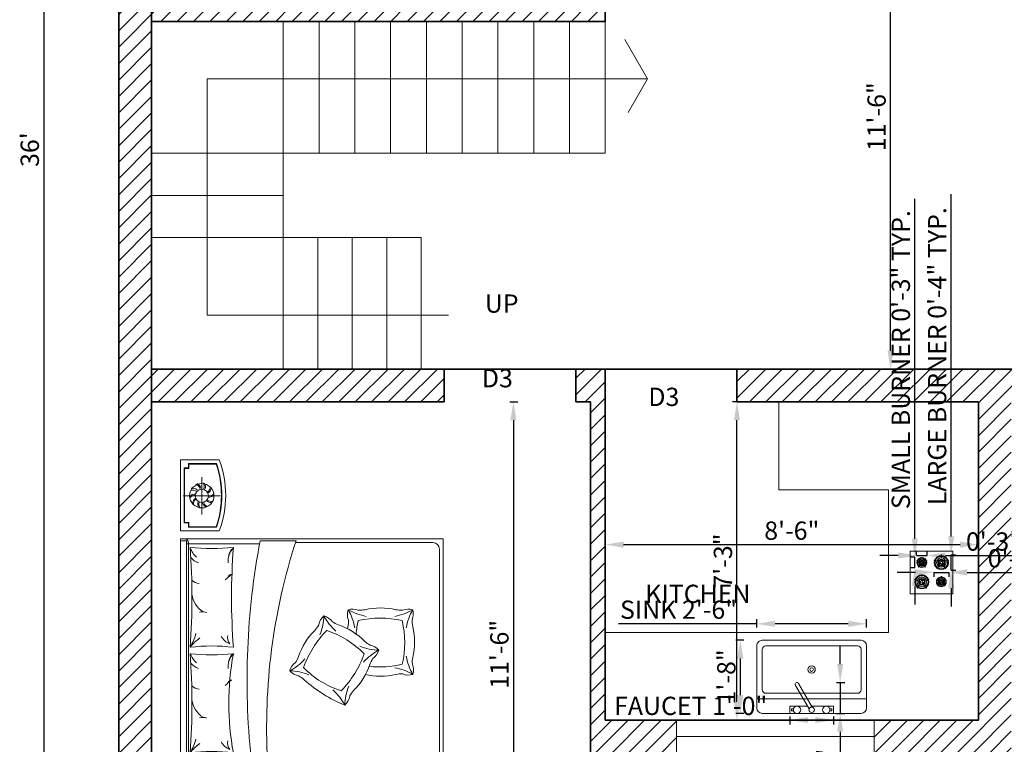
# Model space of a CAD drawing. Units: inches. Extents: x -196 to 219, y -474 to 80.
# Tile 2 of 4: x -196 to 73, y -346 to -148. Entities that reach past the tile are written whole.
import ezdxf

# ---------------------------------------------------------------- set-up
doc = ezdxf.new("R2010")
doc.units = ezdxf.units.IN
doc.header["$PDMODE"] = 35
doc.header["$PDSIZE"] = 5
for name, color, linetype, lineweight in [('A-ANNO-DIMS', 2, 'Continuous', 18), ('A-ANNO-SYMB', 7, 'Continuous', 18), ('A-ANNO-TEXT', 7, 'Continuous', 18), ('A-AREA-IDEN', 7, 'Continuous', 25), ('A-EQPM', 8, 'Continuous', 18), ('A-FLOR-CASE', 34, 'Continuous', 20), ('A-FLOR-FIXT', 9, 'Continuous', 18), ('A-FLOR-STRS', 3, 'Continuous', 18), ('A-GLAZ', 4, 'Continuous', 18), ('A-WALL', 7, 'Continuous', 35), ('A-WALL-PATT', 252, 'Continuous', 13), ('furn', 28, 'Continuous', 18)]:
    doc.layers.add(name, color=color, linetype=linetype, lineweight=lineweight)
doc.styles.get("Standard").update_dxf_attribs({"font": 'arial.ttf'})
doc.dimstyles.new('ISO-25', dxfattribs={"dimtxt": 5, "dimasz": 5, "dimexe": 1.25, "dimexo": 0.625, "dimtad": 1, "dimlunit": 3, "dimtxsty": 'Standard', "dimcen": 2.5, "dimadec": 0, "dimazin": 0, "dimtfac": 1, "dimtmove": 0, "dimatfit": 3, "dimfxl": 1, "dimfxlon": 1, "dimarcsym": 0})

# ---------------------------------------------------------------- blocks, each defined once
blk = doc.blocks.new('*D16')
at = {"layer": 'A-ANNO-DIMS', "color": 0, "lineweight": -2, "transparency": 16777216}
for p, q in [((43.3, -105.09), (41.05, -105.09)), ((42.3, -238.09), (42.3, -110.09)), ((43.3, -243.09), (41.05, -243.09))]:
    blk.add_line(p, q, dxfattribs=at)
at = {"layer": 'A-ANNO-DIMS', "color": 0, "transparency": 16777216}
for points in [[(41.47, -110.09), (43.14, -110.09), (42.3, -105.09)], [(41.47, -238.09), (43.14, -238.09), (42.3, -243.09)]]:
    blk.add_solid(points, dxfattribs=at)
at = {"layer": 'Defpoints', "color": 0, "transparency": 16777216}
for p in [(42.3, -105.09), (44.21, -105.09), (44.21, -243.09)]:
    blk.add_point(p, dxfattribs=at)
at = {"layer": 'A-ANNO-DIMS', "color": 0, "transparency": 16777216, "insert": (39.12, -174.09), "char_height": 5, "attachment_point": 5, "rotation": 90}
blk.add_mtext('11\'-6"', dxfattribs=at)
blk = doc.blocks.new('*D18')
at = {"layer": 'A-ANNO-DIMS', "color": 0, "lineweight": -2, "transparency": 16777216}
for p, q in [((-61.81, -252.09), (-59.56, -252.09)), ((-60.81, -257.09), (-60.81, -385.09)), ((-61.81, -390.09), (-59.56, -390.09))]:
    blk.add_line(p, q, dxfattribs=at)
at = {"layer": 'A-ANNO-DIMS', "color": 0, "transparency": 16777216}
for points in [[(-61.65, -257.09), (-59.98, -257.09), (-60.81, -252.09)], [(-61.65, -385.09), (-59.98, -385.09), (-60.81, -390.09)]]:
    blk.add_solid(points, dxfattribs=at)
at = {"layer": 'Defpoints', "color": 0, "transparency": 16777216}
for p in [(-159.7, -252.09), (-159.7, -390.09), (-60.81, -390.09)]:
    blk.add_point(p, dxfattribs=at)
at = {"layer": 'A-ANNO-DIMS', "color": 0, "transparency": 16777216, "insert": (-63.99, -321.09), "char_height": 5, "attachment_point": 5, "rotation": 90}
blk.add_mtext('11\'-6"', dxfattribs=at)
blk = doc.blocks.new('*D20')
at = {"layer": 'A-ANNO-DIMS', "color": 0, "lineweight": -2, "transparency": 16777216}
for p, q in [((-35.7, -291.09), (-35.7, -289.84)), ((66.3, -291.09), (66.3, -289.84)), ((-30.7, -291.09), (61.3, -291.09))]:
    blk.add_line(p, q, dxfattribs=at)
at = {"layer": 'A-ANNO-DIMS', "color": 0, "transparency": 16777216}
for points in [[(-30.7, -290.26), (-30.7, -291.93), (-35.7, -291.09)], [(61.3, -290.26), (61.3, -291.93), (66.3, -291.09)]]:
    blk.add_solid(points, dxfattribs=at)
at = {"layer": 'Defpoints', "color": 0, "transparency": 16777216}
for p in [(-35.7, -291.09), (66.3, -291.09), (66.3, -291.09)]:
    blk.add_point(p, dxfattribs=at)
at = {"layer": 'A-ANNO-DIMS', "color": 0, "transparency": 16777216, "insert": (15.3, -287.92), "char_height": 5, "attachment_point": 5}
blk.add_mtext('8\'-6"', dxfattribs=at)
blk = doc.blocks.new('*D21')
at = {"layer": 'A-ANNO-DIMS', "color": 0, "lineweight": -2, "transparency": 16777216}
for p, q in [((1.3, -252.09), (-0.95, -252.09)), ((0.3, -334.09), (0.3, -257.09)), ((1.3, -339.09), (-0.95, -339.09))]:
    blk.add_line(p, q, dxfattribs=at)
at = {"layer": 'A-ANNO-DIMS', "color": 0, "transparency": 16777216}
for points in [[(-0.53, -257.09), (1.14, -257.09), (0.3, -252.09)], [(-0.53, -334.09), (1.14, -334.09), (0.3, -339.09)]]:
    blk.add_solid(points, dxfattribs=at)
at = {"layer": 'Defpoints', "color": 0, "transparency": 16777216}
for p in [(0.3, -252.09), (66.3, -252.09), (66.3, -339.09)]:
    blk.add_point(p, dxfattribs=at)
at = {"layer": 'A-ANNO-DIMS', "color": 0, "transparency": 16777216, "insert": (-2.88, -295.59), "char_height": 5, "attachment_point": 5, "rotation": 90}
blk.add_mtext('7\'-3"', dxfattribs=at)
blk = doc.blocks.new('Sink-single - 30 in top')
blk.add_line((-15, -3.999996), (15, -3.999996))
for points in [[(-13.5, 0), (13.5, 0)], [(-15, -18.499996), (-15, -1.5)], [(15, -1.5), (15, -18.499996)], [(-13.5, -17.499996), (-13.5, -6.499996)], [(-12.5, -5.499996), (12.5, -5.499996)], [(13.5, -6.499996), (13.5, -17.499996)], [(12.5, -18.499996), (-12.5, -18.499996)], [(13.5, -19.999996), (-13.5, -19.999996)]]:
    blk.add_lwpolyline(points)
for radius in [1, 0.5]:
    blk.add_circle((0, -11.999996), radius)
for centre, radius, start, end in [((-13.5, -1.5), 1.5, 90, 180), ((13.5, -1.5), 1.5, 0, 90), ((-12.5, -6.499996), 1, 90, 180), ((12.5, -6.499996), 1, 0, 90), ((-13.5, -18.499996), 1.5, 180, 270), ((-12.5, -17.499996), 1, 180, 270), ((12.5, -17.499996), 1, 270, 0), ((13.5, -18.499996), 1.5, 270, 0)]:
    blk.add_arc(centre, radius, start, end)
blk = doc.blocks.new('Faucet - kit sink top')
for p, q in [((-5.5, -0.75), (-5.5, -1.25)), ((-4.94278, -0.75), (-5.5, -0.75)), ((-5.5, -1.25), (-4.94278, -1.25)), ((-0.14775, -1.7441), (3.56698, -8.1782)), ((4.43301, -7.6782), (0.71828, -1.2441)), ((4.94278, -0.75), (5.5, -0.75)), ((5.5, -1.25), (4.94278, -1.25)), ((5.5, -0.75), (5.5, -1.25))]:
    blk.add_line(p, q)
blk.add_lwpolyline([(-0.00587, -2), (-6, -2), (-6, 0), (6, 0), (6, -2), (1.15195, -2)])
for centre, radius in [((-4, -1), 1), ((4, -1), 1), ((0, -1), 0.75)]:
    blk.add_circle(centre, radius)
blk.add_arc((4, -7.9282), 0.5, 210, 30)
blk = doc.blocks.new('*D26')
at = {"layer": 'A-ANNO-DIMS', "color": 0, "lineweight": -2, "transparency": 16777216}
for p, q in [((-188.18, 32.91), (-190.43, 32.91)), ((-189.18, 27.91), (-189.18, -394.09)), ((-188.18, -399.09), (-190.43, -399.09))]:
    blk.add_line(p, q, dxfattribs=at)
at = {"layer": 'A-ANNO-DIMS', "color": 0, "transparency": 16777216}
for points in [[(-190.01, 27.91), (-188.35, 27.91), (-189.18, 32.91)], [(-190.01, -394.09), (-188.35, -394.09), (-189.18, -399.09)]]:
    blk.add_solid(points, dxfattribs=at)
at = {"layer": 'Defpoints', "color": 0, "transparency": 16777216}
for p in [(-168.7, 32.91), (-189.18, -399.09), (-168.7, -399.09)]:
    blk.add_point(p, dxfattribs=at)
at = {"layer": 'A-ANNO-DIMS', "color": 0, "transparency": 16777216, "insert": (-192.36, -183.09), "char_height": 5, "attachment_point": 5, "rotation": 90}
blk.add_mtext("36'", dxfattribs=at)
blk = doc.blocks.new('BED-DOUBLE')
for p, q in [((70.2, 59.88), (52.52, 59.88)), ((69.67, 60.18), (69.67, 1.06)), ((70.2, 1.4), (50.22, 1.4))]:
    blk.add_line(p, q)
for points in [[(71.86, 61.24), (0, 61.24), (0, 0), (71.86, 0)], [(71.86, 0.57), (70.2, 0.57), (70.2, 60.89), (71.86, 60.89), (71.86, 0)]]:
    blk.add_lwpolyline(points)
for points in [[(48.05, 60.18), (2.83, 60.18, 0.414214), (1.06, 58.41), (1.06, 2.83, 0.414214), (2.83, 1.06), (40.4, 1.06)], [(25.84, 40.29, 0.091296), (26.93, 45.48, 0.091296), (30.19, 41.3, 0.091296)], [(27.91, 41.58, 0.111006), (21.62, 31.47, 0.119549), (31.85, 25.09, 0.107813), (38.17, 35.17)], [(38.16, 35.23, 0.121865), (27.91, 41.58, 0.121865)], [(10.11, 32.11, 0.091296), (8.3, 37.09, 0.091296), (13.27, 35.26, 0.091296)], [(36.77, 37.19, 0.091296), (41.96, 36.12, 0.091296), (37.79, 32.85, 0.091296)], [(11.19, 34.3, 0.111006), (11.2, 22.39, 0.119549), (23.25, 22.39, 0.033212), (23.81, 26.05)], [(22.76, 29.38, 0.091296), (17.57, 30.45, 0.091296), (21.75, 33.72)], [(17.57, 30.45, 0.159461), (20.01, 29.08, -0.076283), (21.52, 28, 0.115075), (28.65, 23.55, -0.076283), (30.29, 22.67, 0.159461), (32.6, 21.09)], [(13.27, 21.22, 0.091296), (8.3, 19.39, 0.091296), (10.11, 24.37)], [(24.18, 24.37, 0.091296), (26, 19.39, 0.091296), (21.02, 21.22, 0.091296)], [(33.69, 26.28, 0.091296), (32.6, 21.09, 0.091296), (29.35, 25.28, 0.091296)], [(8.3, 19.39, 0.159461), (11.08, 19.51, -0.076283), (12.94, 19.39, 0.115075), (21.35, 19.39, -0.076283), (23.21, 19.51, 0.159461), (26, 19.39)]]:
    blk.add_lwpolyline(points, format="xyb")
for points in [[(52.52, 60.71), (52.52, 59.88, -0.072944), (50.05, 0.57), (40.23, 0.57, 0.092568), (48.02, 60.71)], [(57.36, 58.53, 0.058596), (69.19, 58.53, 0.036889), (69.19, 31.42, 0.052163), (57.36, 31.42, 0.093111)], [(57.36, 29.66, 0.058596), (69.19, 29.66, 0.036648), (69.19, 2.37, 0.052163), (57.36, 2.37, 0.036967)]]:
    blk.add_lwpolyline(points, format="xyb", close=True)
for centre, radius, start, end in [((70.74, 60.18), 1.06, 90, 180), ((56.26, 55.91), 2.69, 346.4823, 38.5563), ((57.08, 53.87), 3.93, 24.2916, 70.9896), ((58.12, 67.4), 14.18, 306.4935, 321.2792), ((79.08, 52.23), 11.72, 147.5379, 167.5233), ((65.82, 51.76), 2.94, 245.8927, 286.1192), ((62.17, 43.24), 6.56, 6.6849, 58.3182), ((29.97, 42.18), 4.49, 132.6522, 168.8929), ((12.27, 9.6), 38.76, 48.3818, 67.7644), ((37.6, 28.47), 18.5, 135.1307, 161.3884), ((20.09, 45.81), 6.15, 315.7718, 333.2208), ((65.9, 36.61), 4.6, 51.8174, 79.8987), ((42.31, 42.96), 6.15, 225.5854, 243.0343), ((57.86, 39.62), 0.992, 263.7543, 347.2187), ((49.13, 50.55), 14.78, 306.2085, 315.0849), ((12.62, 35.9), 4.49, 164.5791, 200.8198), ((9.5, 32.77), 4.49, 69.3666, 105.6073), ((11.62, 43.09), 6.15, 265.0387, 282.4877), ((17.27, 9.95), 25.09, 83.1956, 104.0284), ((17.15, 19.08), 18.5, 76.8711, 103.1289), ((38.65, 33.09), 4.49, 42.4658, 78.7065), ((37.79, 37.3), 4.33, 307.2937, 344.0973), ((53.97, 34.88), 4.84, 314.406, 6.8342), ((65.25, 30.79), 4.95, 40.5354, 70.3558), ((26.34, 28.3), 18.5, 167.0576, 193.3153), ((2.31, 33.75), 6.15, 347.6988, 5.1477), ((22.41, 28.73), 5.13, 128.7754, 160.3571), ((14.27, 36.4), 6.15, 323.2983, 340.7472), ((45.34, 30.19), 6.15, 143.2983, 160.7472), ((55.66, 33.97), 3.07, 303.6349, 0.8456), ((61.08, 27.7), 8.92, 24.6457, 44.1585), ((22.01, 38.11), 18.5, 315.1307, 341.3884), ((58.12, 38.53), 14.18, 306.4935, 321.2792), ((79.08, 23.37), 11.72, 147.5379, 167.5233), ((56.26, 27.04), 2.69, 346.4823, 38.5563), ((57.08, 25), 3.93, 24.2916, 70.9896), ((8.01, 28.24), 18.5, 347.0576, 348.7033), ((39.53, 20.78), 6.15, 135.7718, 153.2208), ((13.31, 20.48), 5.13, 160.7023, 192.284), ((2.34, 22.69), 6.15, 355.2252, 12.6741), ((32.04, 22.79), 6.15, 167.6988, 185.1477), ((22.07, 20.71), 4.14, 341.3996, 21.5774), ((29.96, 24.29), 4.14, 309.4726, 349.6505), ((65.82, 22.89), 2.94, 245.8927, 286.1192), ((62.17, 14.37), 6.56, 6.6849, 58.3182), ((49.13, 21.68), 14.78, 306.2085, 315.0849), ((65.9, 7.74), 4.6, 51.8174, 79.8987), ((57.86, 10.75), 0.992, 263.7543, 347.2187), ((53.97, 6.01), 4.84, 314.406, 6.8342), ((65.25, 1.92), 4.95, 40.5354, 70.3558), ((55.66, 5.1), 3.07, 303.6349, 0.8456), ((61.08, -1.17), 8.92, 24.6457, 44.1585), ((70.74, 1.06), 1.06, 180, 270)]:
    blk.add_arc(centre, radius, start, end)
blk = doc.blocks.new('NIGHTSTAND-A')
for p, q in [((6.52, 4.73), (6.52, 14.94)), ((1.42, 9.84), (11.63, 9.84))]:
    blk.add_line(p, q)
blk.add_lwpolyline([(1.77, 0), (12.39, 0), (12.39, 19.47), (1.77, 19.47, 0.181818)], format="xyb", close=True)
for points in [[(10.16, 18.41), (2.51, 18.41, 0.167087), (2.51, 1.06), (10.16, 1.06)], [(10.16, 18.3), (2.59, 18.3, 0.165559), (2.59, 1.17), (10.16, 1.17)]]:
    blk.add_lwpolyline(points, format="xyb")
for points in [[(11.33, 17.13), (10.05, 17.13), (10.05, 18.41)], [(11.33, 17.24), (10.16, 17.24), (10.16, 18.41)], [(11.22, 2.23), (11.22, 17.24)], [(11.33, 2.23), (11.33, 17.24)], [(11.33, 2.34), (10.05, 2.34), (10.05, 1.06)], [(11.33, 2.23), (10.16, 2.23), (10.16, 1.06)]]:
    blk.add_lwpolyline(points)
for radius in [3.33, 1.81]:
    blk.add_circle((6.52, 9.84), radius)
for centre, radius, start, end in [((4.07, 9.75), 1.63, 49.462, 109.6998), ((4.02, 9.54), 2.14, 51.5103, 97.83), ((4.49, 11.21), 1.63, 13.462, 73.6998), ((4.33, 11.07), 2.14, 15.5103, 61.83), ((5.68, 12.14), 1.63, 337.462, 37.6998), ((5.47, 12.12), 2.14, 339.5103, 25.83), ((7.2, 12.19), 1.63, 301.462, 1.6998), ((7.01, 12.3), 2.14, 303.5103, 349.83), ((4.68, 8.13), 2.14, 87.5103, 133.83), ((4.59, 8.33), 1.63, 85.462, 145.6998), ((6.03, 7.37), 2.14, 123.5103, 169.83), ((5.85, 7.48), 1.63, 121.462, 181.6998), ((9.11, 9.89), 2.14, 231.5103, 277.83), ((8.97, 9.92), 1.63, 229.462, 289.6998), ((8.37, 11.54), 2.14, 267.5103, 313.83), ((8.45, 11.35), 1.63, 265.462, 325.6998), ((7.67, 7.31), 2.14, 159.5103, 205.83), ((7.45, 7.29), 1.63, 157.462, 217.6998), ((8.81, 8.36), 2.14, 195.5103, 241.83), ((8.65, 8.22), 1.63, 193.462, 253.6998)]:
    blk.add_arc(centre, radius, start, end)
blk = doc.blocks.new('WIN-54IN')
for p, q in [((0, 9), (0, 0)), ((54, 9), (54, 0)), ((0, 4.5), (54, 4.5))]:
    blk.add_line(p, q)
blk = doc.blocks.new('COOKTOP-BURNER-LARGE')
for p, q in [((2, 3.24), (2, 4.03)), ((2.07, 3.24), (2.07, 4.03)), ((0.77, 2.3), (0.02, 2.54)), ((0.79, 2.36), (0.04, 2.61)), ((1.23, 0.88), (0.77, 0.24)), ((1.29, 0.84), (0.82, 0.2)), ((2.78, 0.84), (3.24, 0.2)), ((2.83, 0.88), (3.3, 0.24)), ((3.27, 2.36), (4.02, 2.61)), ((3.29, 2.3), (4.04, 2.54))]:
    blk.add_line(p, q)
for radius in [1.28, 0.919, 0.748, 0.321]:
    blk.add_circle((2.03, 1.92), radius)
for centre, radius, start, end in [((2.03, 1.92), 1.92, 90.9557, 161.0457), ((2.03, 1.92), 1.71, 91.075, 160.9263), ((2.03, 4.03), 0.0321, 0.0007, 180.0007), ((2.03, 3.24), 0.0321, 180.0007, 0.0007), ((2.03, 1.92), 1.92, 18.9557, 89.0457), ((2.03, 1.92), 1.71, 19.075, 88.9263), ((0.03, 2.57), 0.0321, 72.0007, 252.0007), ((2.03, 1.92), 1.92, 162.9557, 233.0457), ((2.03, 1.92), 1.71, 163.075, 232.9263), ((0.8, 0.22), 0.0321, 144.0007, 324.0007), ((0.78, 2.33), 0.0321, 252.0007, 72.0007), ((2.03, 1.92), 1.92, 234.9557, 305.0457), ((2.03, 1.92), 1.71, 235.075, 304.9263), ((1.26, 0.86), 0.0321, 324.0007, 144.0007), ((1.5, 1.92), 0.107, 0.0007, 180.0007), ((2.03, 1.92), 0.641, 180.0007, 213.5265), ((1.59, 1.63), 0.107, 213.5265, 33.5265), ((2.03, 1.92), 0.428, 180.0007, 213.5265), ((2, 2.46), 0.107, 93.5265, 273.5265), ((2.03, 1.92), 0.641, 60.0007, 93.5265), ((2.03, 1.92), 0.428, 60.0007, 93.5265), ((2.3, 1.46), 0.107, 120.0007, 300.0007), ((2.3, 2.39), 0.107, 240.0007, 60.0007), ((2.03, 1.92), 0.428, 300.0007, 333.5265), ((2.03, 1.92), 0.641, 300.0007, 333.5265), ((2.51, 1.69), 0.107, 333.5265, 153.5265), ((2.81, 0.86), 0.0321, 36.0007, 216.0007), ((2.03, 1.92), 1.71, 307.075, 16.9263), ((2.03, 1.92), 1.92, 306.9557, 17.0457), ((3.27, 0.22), 0.0321, 216.0007, 36.0007), ((3.28, 2.33), 0.0321, 108.0007, 288.0007), ((4.03, 2.57), 0.0321, 288.0007, 108.0007)]:
    blk.add_arc(centre, radius, start, end)
blk = doc.blocks.new('COOKTOP-BURNER-SMALL')
for p, q in [((1.4, 2.27), (1.4, 2.82)), ((1.45, 2.27), (1.45, 2.82)), ((0.54, 1.61), (0.02, 1.78)), ((0.55, 1.65), (0.03, 1.82)), ((0.86, 0.62), (0.54, 0.17)), ((0.9, 0.59), (0.58, 0.14)), ((1.95, 0.59), (2.27, 0.14)), ((1.98, 0.62), (2.31, 0.17)), ((2.29, 1.65), (2.82, 1.82)), ((2.31, 1.61), (2.83, 1.78))]:
    blk.add_line(p, q)
for radius in [0.898, 0.644, 0.524, 0.224]:
    blk.add_circle((1.42, 1.35), radius)
for centre, radius, start, end in [((1.42, 1.35), 1.35, 90.9557, 161.0457), ((1.42, 2.82), 0.0224, 0.0007, 180.0007), ((1.42, 1.35), 1.35, 18.9557, 89.0457), ((0.02, 1.8), 0.0224, 72.0007, 252.0007), ((1.42, 1.35), 1.35, 162.9557, 233.0457), ((1.42, 1.35), 1.2, 163.075, 232.9263), ((1.42, 1.35), 1.2, 91.075, 160.9263), ((0.56, 0.15), 0.0224, 144.0007, 324.0007), ((0.55, 1.63), 0.0224, 252.0007, 72.0007), ((1.37, 1.35), 1.35, 234.9557, 305.0457), ((1.42, 1.35), 1.2, 235.075, 304.9263), ((0.88, 0.6), 0.0224, 324.0007, 144.0007), ((1.09, 1.18), 0.0748, 26.4748, 206.4748), ((1.42, 1.35), 0.449, 206.4748, 240.0007), ((1.24, 1.67), 0.0748, 120.0007, 300.0007), ((1.42, 1.35), 0.299, 206.4748, 240.0007), ((1.42, 1.35), 0.449, 86.4748, 120.0007), ((1.24, 1.02), 0.0748, 240.0007, 60.0007), ((1.42, 1.35), 0.299, 86.4748, 120.0007), ((1.42, 2.27), 0.0224, 180.0007, 0.0007), ((1.45, 1.72), 0.0748, 266.4748, 86.4748), ((1.42, 1.35), 1.2, 19.075, 88.9263), ((1.74, 1.14), 0.0748, 146.4748, 326.4748), ((1.42, 1.35), 0.299, 326.4748, 0.0007), ((1.8, 1.35), 0.0748, 0.0007, 180.0007), ((1.42, 1.35), 0.449, 326.4748, 0.0007), ((1.96, 0.6), 0.0224, 36.0007, 216.0007), ((1.42, 1.35), 1.2, 307.075, 16.9263), ((1.42, 1.35), 1.35, 306.9557, 17.0457), ((2.29, 0.15), 0.0224, 216.0007, 36.0007), ((2.3, 1.63), 0.0224, 108.0007, 288.0007), ((2.82, 1.8), 0.0224, 288.0007, 108.0007)]:
    blk.add_arc(centre, radius, start, end)
blk = doc.blocks.new('*D48')
at = {"layer": 'A-ANNO-DIMS', "color": 0, "lineweight": -2, "transparency": 16777216}
for p, q in [((58.88, -288.86), (58.88, -195.3)), ((58.88, -293.86), (60.13, -293.86)), ((58.88, -298.04), (58.88, -293.86)), ((58.88, -298.04), (60.13, -298.04)), ((58.88, -303.04), (58.88, -308.04))]:
    blk.add_line(p, q, dxfattribs=at)
at = {"layer": 'A-ANNO-DIMS', "color": 0, "transparency": 16777216}
for points in [[(58.04, -288.86), (59.71, -288.86), (58.88, -293.86)], [(58.04, -303.04), (59.71, -303.04), (58.88, -298.04)]]:
    blk.add_solid(points, dxfattribs=at)
at = {"layer": 'Defpoints', "color": 0, "transparency": 16777216}
for p in [(58.25, -293.86), (58.88, -293.86), (58.25, -298.04)]:
    blk.add_point(p, dxfattribs=at)
at = {"layer": 'A-ANNO-DIMS', "color": 0, "transparency": 16777216, "insert": (55.67, -239.58), "char_height": 5, "attachment_point": 5, "rotation": 90}
blk.add_mtext('LARGE BURNER 0\'-4" TYP.', dxfattribs=at)
blk = doc.blocks.new('*D49')
at = {"layer": 'A-ANNO-DIMS', "color": 0, "lineweight": -2, "transparency": 16777216}
for p, q in [((49.1, -298.67), (44.1, -298.67)), ((54.1, -298.67), (54.1, -299.92)), ((54.1, -298.67), (58.25, -298.67)), ((58.25, -298.67), (58.25, -299.92)), ((63.25, -298.67), (99.98, -298.67))]:
    blk.add_line(p, q, dxfattribs=at)
at = {"layer": 'A-ANNO-DIMS', "color": 0, "transparency": 16777216}
for points in [[(49.1, -297.83), (49.1, -299.5), (54.1, -298.67)], [(63.25, -297.83), (63.25, -299.5), (58.25, -298.67)]]:
    blk.add_solid(points, dxfattribs=at)
at = {"layer": 'Defpoints', "color": 0, "transparency": 16777216}
for p in [(54.1, -298.04), (58.25, -298.04), (58.25, -298.67)]:
    blk.add_point(p, dxfattribs=at)
at = {"layer": 'A-ANNO-DIMS', "color": 0, "transparency": 16777216, "insert": (84.11, -295.49), "char_height": 5, "attachment_point": 5}
blk.add_mtext('0\'-4" TYP.', dxfattribs=at)
blk = doc.blocks.new('*D50')
at = {"layer": 'A-ANNO-DIMS', "color": 0, "lineweight": -2, "transparency": 16777216}
for p, q in [((48.95, -289.5), (48.95, -196.52)), ((48.95, -294.5), (47.7, -294.5)), ((48.95, -297.43), (48.95, -294.5)), ((48.95, -297.43), (47.7, -297.43)), ((48.95, -302.43), (48.95, -307.43))]:
    blk.add_line(p, q, dxfattribs=at)
at = {"layer": 'A-ANNO-DIMS', "color": 0, "transparency": 16777216}
for points in [[(48.12, -289.5), (49.78, -289.5), (48.95, -294.5)], [(48.12, -302.43), (49.78, -302.43), (48.95, -297.43)]]:
    blk.add_solid(points, dxfattribs=at)
at = {"layer": 'Defpoints', "color": 0, "transparency": 16777216}
for p in [(48.95, -294.5), (49.39, -294.5), (49.39, -297.43)]:
    blk.add_point(p, dxfattribs=at)
at = {"layer": 'A-ANNO-DIMS', "color": 0, "transparency": 16777216, "insert": (45.74, -240.51), "char_height": 5, "attachment_point": 5, "rotation": 90}
blk.add_mtext('SMALL BURNER 0\'-3" TYP.', dxfattribs=at)
blk = doc.blocks.new('*D51')
at = {"layer": 'A-ANNO-DIMS', "color": 0, "lineweight": -2, "transparency": 16777216}
for p, q in [((49.39, -294.07), (49.39, -292.82)), ((52.3, -294.07), (52.3, -292.82)), ((44.39, -294.07), (39.39, -294.07)), ((49.39, -294.07), (52.3, -294.07)), ((57.3, -294.07), (94.02, -294.07))]:
    blk.add_line(p, q, dxfattribs=at)
at = {"layer": 'A-ANNO-DIMS', "color": 0, "transparency": 16777216}
for points in [[(44.39, -293.23), (44.39, -294.9), (49.39, -294.07)], [(57.3, -293.23), (57.3, -294.9), (52.3, -294.07)]]:
    blk.add_solid(points, dxfattribs=at)
at = {"layer": 'Defpoints', "color": 0, "transparency": 16777216}
for p in [(49.39, -294.5), (52.3, -294.07), (52.3, -294.5)]:
    blk.add_point(p, dxfattribs=at)
at = {"layer": 'A-ANNO-DIMS', "color": 0, "transparency": 16777216, "insert": (78.16, -290.89), "char_height": 5, "attachment_point": 5}
blk.add_mtext('0\'-3" TYP.', dxfattribs=at)
blk = doc.blocks.new('*D52')
at = {"layer": 'A-ANNO-DIMS', "color": 0, "lineweight": -2, "transparency": 16777216}
for p, q in [((5.72, -313.75), (5.72, -311.5)), ((35.72, -313.75), (35.72, -311.5)), ((5.72, -312.75), (-32.04, -312.75)), ((30.72, -312.75), (10.72, -312.75))]:
    blk.add_line(p, q, dxfattribs=at)
at = {"layer": 'A-ANNO-DIMS', "color": 0, "transparency": 16777216}
for points in [[(10.72, -311.91), (10.72, -313.58), (5.72, -312.75)], [(30.72, -311.91), (30.72, -313.58), (35.72, -312.75)]]:
    blk.add_solid(points, dxfattribs=at)
at = {"layer": 'Defpoints', "color": 0, "transparency": 16777216}
for p in [(5.72, -312.75), (5.72, -317.25), (35.72, -317.25)]:
    blk.add_point(p, dxfattribs=at)
at = {"layer": 'A-ANNO-DIMS', "color": 0, "transparency": 16777216, "insert": (-15.66, -309.53), "char_height": 5, "attachment_point": 5}
blk.add_mtext('SINK 2\'-6"', dxfattribs=at)
blk = doc.blocks.new('*D53')
at = {"layer": 'A-ANNO-DIMS', "color": 0, "lineweight": -2, "transparency": 16777216}
for p, q in [((2.22, -317.25), (-0.03, -317.25)), ((1.22, -322.25), (1.22, -332.25)), ((2.22, -337.25), (-0.03, -337.25))]:
    blk.add_line(p, q, dxfattribs=at)
at = {"layer": 'A-ANNO-DIMS', "color": 0, "transparency": 16777216}
for points in [[(0.39, -322.25), (2.06, -322.25), (1.22, -317.25)], [(0.39, -332.25), (2.06, -332.25), (1.22, -337.25)]]:
    blk.add_solid(points, dxfattribs=at)
at = {"layer": 'Defpoints', "color": 0, "transparency": 16777216}
for p in [(5.72, -317.25), (1.22, -337.25), (5.72, -337.25)]:
    blk.add_point(p, dxfattribs=at)
at = {"layer": 'A-ANNO-DIMS', "color": 0, "transparency": 16777216, "insert": (-1.95, -327.25), "char_height": 5, "attachment_point": 5, "rotation": 90}
blk.add_mtext('1\'-8"', dxfattribs=at)
blk = doc.blocks.new('*D54')
at = {"layer": 'A-ANNO-DIMS', "color": 0, "lineweight": -2, "transparency": 16777216}
for p, q in [((14.72, -339.05), (-34.42, -339.05)), ((14.72, -338.05), (14.72, -340.3)), ((21.72, -339.05), (19.72, -339.05)), ((26.72, -338.05), (26.72, -340.3))]:
    blk.add_line(p, q, dxfattribs=at)
at = {"layer": 'A-ANNO-DIMS', "color": 0, "transparency": 16777216}
for points in [[(19.72, -338.21), (19.72, -339.88), (14.72, -339.05)], [(21.72, -338.21), (21.72, -339.88), (26.72, -339.05)]]:
    blk.add_solid(points, dxfattribs=at)
at = {"layer": 'Defpoints', "color": 0, "transparency": 16777216}
for p in [(14.72, -337.25), (14.72, -339.05), (26.72, -337.25)]:
    blk.add_point(p, dxfattribs=at)
at = {"layer": 'A-ANNO-DIMS', "color": 0, "transparency": 16777216, "insert": (-12.35, -335.83), "char_height": 5, "attachment_point": 5}
blk.add_mtext('FAUCET 1\'-0"', dxfattribs=at)
blk = doc.blocks.new('*D55')
at = {"layer": 'A-ANNO-DIMS', "color": 0, "lineweight": -2, "transparency": 16777216}
for p, q in [((28.52, -323.75), (28.52, -318.75)), ((27.52, -328.75), (29.77, -328.75)), ((28.52, -328.75), (28.52, -337.25)), ((27.52, -337.25), (29.77, -337.25)), ((28.52, -342.25), (28.52, -373.44))]:
    blk.add_line(p, q, dxfattribs=at)
at = {"layer": 'A-ANNO-DIMS', "color": 0, "transparency": 16777216}
for points in [[(27.69, -323.75), (29.36, -323.75), (28.52, -328.75)], [(27.69, -342.25), (29.36, -342.25), (28.52, -337.25)]]:
    blk.add_solid(points, dxfattribs=at)
at = {"layer": 'Defpoints', "color": 0, "transparency": 16777216}
for p in [(26.72, -328.75), (26.72, -337.25), (28.52, -337.25)]:
    blk.add_point(p, dxfattribs=at)
at = {"layer": 'A-ANNO-DIMS', "color": 0, "transparency": 16777216, "insert": (25.31, -360.34), "char_height": 5, "attachment_point": 5, "rotation": 90}
blk.add_mtext('0\'-8 1/2"', dxfattribs=at)
blk = doc.blocks.new('*D56')
at = {"layer": 'A-ANNO-DIMS', "color": 0, "lineweight": -2, "transparency": 16777216}
for p, q in [((216.25, -148.09), (218.5, -148.09)), ((217.25, -153.09), (217.25, -179.09)), ((216.25, -184.09), (218.5, -184.09))]:
    blk.add_line(p, q, dxfattribs=at)
at = {"layer": 'A-ANNO-DIMS', "color": 0, "transparency": 16777216}
for points in [[(216.42, -153.09), (218.09, -153.09), (217.25, -148.09)], [(216.42, -179.09), (218.09, -179.09), (217.25, -184.09)]]:
    blk.add_solid(points, dxfattribs=at)
at = {"layer": 'Defpoints', "color": 0, "transparency": 16777216}
for p in [(-35.7, -148.09), (-35.7, -184.09), (217.25, -184.09)]:
    blk.add_point(p, dxfattribs=at)
at = {"layer": 'A-ANNO-DIMS', "color": 0, "transparency": 16777216, "insert": (214.07, -166.09), "char_height": 5, "attachment_point": 5, "rotation": 90}
blk.add_mtext('3\'-0"', dxfattribs=at)
blk = doc.blocks.new('*D57')
at = {"layer": 'A-ANNO-DIMS', "color": 0, "lineweight": -2, "transparency": 16777216}
for p, q in [((-35.7, -454.04), (-35.7, -456.29)), ((0.3, -454.04), (0.3, -456.29)), ((-30.7, -455.04), (-4.7, -455.04))]:
    blk.add_line(p, q, dxfattribs=at)
at = {"layer": 'A-ANNO-DIMS', "color": 0, "transparency": 16777216}
for points in [[(-30.7, -454.21), (-30.7, -455.88), (-35.7, -455.04)], [(-4.7, -454.21), (-4.7, -455.88), (0.3, -455.04)]]:
    blk.add_solid(points, dxfattribs=at)
at = {"layer": 'Defpoints', "color": 0, "transparency": 16777216}
for p in [(-35.7, -243.09), (0.3, -243.09), (0.3, -455.04)]:
    blk.add_point(p, dxfattribs=at)
at = {"layer": 'A-ANNO-DIMS', "color": 0, "transparency": 16777216, "insert": (-17.7, -451.86), "char_height": 5, "attachment_point": 5}
blk.add_mtext('3\'-0"', dxfattribs=at)
blk = doc.blocks.new('*D58')
at = {"layer": 'A-ANNO-DIMS', "color": 0, "lineweight": -2, "transparency": 16777216}
for p, q in [((-21.7, -454.04), (-21.7, -456.29)), ((8.3, -454.04), (8.3, -456.29)), ((-16.7, -455.04), (3.3, -455.04))]:
    blk.add_line(p, q, dxfattribs=at)
at = {"layer": 'A-ANNO-DIMS', "color": 0, "transparency": 16777216}
for points in [[(-16.7, -454.21), (-16.7, -455.88), (-21.7, -455.04)], [(3.3, -454.21), (3.3, -455.88), (8.3, -455.04)]]:
    blk.add_solid(points, dxfattribs=at)
at = {"layer": 'Defpoints', "color": 0, "transparency": 16777216}
for p in [(-21.7, -60.09), (8.3, -64.09), (8.3, -455.04)]:
    blk.add_point(p, dxfattribs=at)
at = {"layer": 'A-ANNO-DIMS', "color": 0, "transparency": 16777216, "insert": (-6.7, -451.87), "char_height": 5, "attachment_point": 5}
blk.add_mtext('2\'-6"', dxfattribs=at)
blk = doc.blocks.new('*D60')
at = {"layer": 'A-ANNO-DIMS', "color": 0, "lineweight": -2, "transparency": 16777216}
for p, q in [((61.3, 73.61), (56.3, 73.61)), ((66.3, 72.61), (66.3, 74.86)), ((66.3, 73.61), (75.3, 73.61)), ((75.3, 72.61), (75.3, 74.86)), ((80.3, 73.61), (99.84, 73.61))]:
    blk.add_line(p, q, dxfattribs=at)
at = {"layer": 'A-ANNO-DIMS', "color": 0, "transparency": 16777216}
for points in [[(61.3, 74.45), (61.3, 72.78), (66.3, 73.61)], [(80.3, 74.45), (80.3, 72.78), (75.3, 73.61)]]:
    blk.add_solid(points, dxfattribs=at)
at = {"layer": 'Defpoints', "color": 0, "transparency": 16777216}
for p in [(75.3, 73.61), (66.3, -339.09), (75.3, -348.09)]:
    blk.add_point(p, dxfattribs=at)
at = {"layer": 'A-ANNO-DIMS', "color": 0, "transparency": 16777216, "insert": (92.57, 76.79), "char_height": 5, "attachment_point": 5}
blk.add_mtext('0\'-9"', dxfattribs=at)
blk = doc.blocks.new('*D61')
at = {"layer": 'A-ANNO-DIMS', "color": 0, "lineweight": -2, "transparency": 16777216}
for p, q in [((-39.7, -454.04), (-39.7, -456.29)), ((-35.7, -454.04), (-35.7, -456.29)), ((-44.7, -455.04), (-49.7, -455.04)), ((-39.7, -455.04), (-35.7, -455.04)), ((-30.7, -455.04), (-11.16, -455.04))]:
    blk.add_line(p, q, dxfattribs=at)
at = {"layer": 'A-ANNO-DIMS', "color": 0, "transparency": 16777216}
for points in [[(-44.7, -454.21), (-44.7, -455.88), (-39.7, -455.04)], [(-30.7, -454.21), (-30.7, -455.88), (-35.7, -455.04)]]:
    blk.add_solid(points, dxfattribs=at)
at = {"layer": 'Defpoints', "color": 0, "transparency": 16777216}
for p in [(-35.7, -243.09), (-39.7, -252.09), (-35.7, -455.04)]:
    blk.add_point(p, dxfattribs=at)
at = {"layer": 'A-ANNO-DIMS', "color": 0, "transparency": 16777216, "insert": (-18.43, -451.87), "char_height": 5, "attachment_point": 5}
blk.add_mtext('0\'-4"', dxfattribs=at)

msp = doc.modelspace()

# ---------------------------------------------------------------- hatches: boundary and pattern name
at = {"layer": 'A-WALL-PATT'}
h = msp.add_hatch(dxfattribs=at)
h.set_pattern_fill('ANSI31', color=256)
h.set_pattern_definition([(45, (-560.5042, 72.7454), (-2.245064, 2.245064), [])])
h.paths.add_polyline_path([(-159.698, -243.094), (-159.698, -148.094), (-159.698, 23.906), (-39.698, 23.906), (-39.698, -108.969), (-35.698, -108.969), (-35.698, -105.094), (-23.894, -105.094), (-23.894, -96.094), (-35.698, -96.094), (-35.698, -64.094), (-21.698, -64.094), (-21.698, -60.094), (-35.698, -60.094), (-35.698, -12.094), (-24.951, -12.094), (-24.951, -8.094), (-35.698, -8.094), (-35.698, 23.906), (-35.698, 27.906), (60.302, 27.906), (60.302, 23.906), (60.302, -8.094), (42.302, -8.094), (42.302, -12.094), (60.302, -12.094), (60.302, -96.094), (42.302, -96.094), (8.302, -96.094), (8.302, -105.094), (42.302, -105.094), (60.302, -105.094), (64.302, -105.094), (64.302, 23.906), (182.302, 23.906), (182.302, -96.094), (100.302, -96.094), (100.302, -105.094), (182.302, -105.094), (182.302, -252.094), (191.302, -252.094), (191.302, 32.906), (-168.698, 32.906), (-168.698, -399.094), (-134.786, -399.094), (-134.786, -390.094), (-159.698, -390.094)])
h.paths.add_polyline_path([(191.302, -252.094), (187.302, -252.094), (187.302, -420.094), (183.555, -420.094), (183.555, -429.094), (191.302, -429.094)])
h.paths.add_polyline_path([(87.555, -420.094), (75.302, -420.094), (38.543, -420.094), (3.06, -420.094), (3.06, -425.094), (3.06, -429.094), (87.555, -429.094)])
h.paths.add_polyline_path([(75.302, -252.094), (81.302, -252.094), (81.302, -243.094), (0.302, -243.094), (0.302, -252.094), (66.302, -252.094), (66.302, -339.094), (37.784, -339.094), (37.784, -348.094), (66.302, -348.094), (75.302, -348.094)], flags=17)
h.paths.add_polyline_path([(-16.216, -339.094), (-35.698, -339.094), (-35.698, -243.094), (-43.698, -243.094), (-43.698, -252.094), (-39.698, -252.094), (-39.698, -352.094), (-35.698, -352.094), (-35.698, -348.094), (-16.216, -348.094)], flags=17)
h.paths.add_polyline_path([(-79.698, -243.094), (-159.698, -243.094), (-159.698, -252.094), (-79.698, -252.094)], flags=17)
h.paths.add_polyline_path([(-35.698, -144.094), (-159.698, -144.094), (-159.698, -148.094), (-35.698, -148.094)], flags=17)

# ---------------------------------------------------------------- linework, layer by layer
at = {"layer": 'A-ANNO-SYMB'}
for p, q in [((-24.108, -163.766), (-30.321, -153.006)), ((-144.551, -228.382), (-144.551, -163.766)), ((-144.551, -163.766), (-24.108, -163.766)), ((-24.108, -163.766), (-29.424, -172.974)), ((-78.536, -228.382), (-144.551, -228.382))]:
    msp.add_line(p, q, dxfattribs=at)
at = {"layer": 'A-EQPM'}
msp.add_lwpolyline([(47.677, -304.504), (59.339, -304.504), (59.339, -292.842), (47.677, -292.842)], close=True, dxfattribs=at)
at = {"layer": 'A-FLOR-CASE'}
for p, q in [((11.763, -252.094), (11.763, -276.094)), ((11.763, -276.094), (41.76, -276.094)), ((41.76, -276.094), (41.76, -315.094)), ((-35.698, -315.094), (41.76, -315.094))]:
    msp.add_line(p, q, dxfattribs=at)
at = {"layer": 'A-FLOR-STRS'}
for p, q in [((-123.698, -243.094), (-123.698, -148.094)), ((-123.698, -148.094), (-123.698, -184.094)), ((-113.92, -148.094), (-113.92, -184.094)), ((-104.142, -148.094), (-104.142, -184.094)), ((-94.365, -148.094), (-94.365, -184.094)), ((-84.587, -148.094), (-84.587, -184.094)), ((-74.809, -148.094), (-74.809, -184.094)), ((-65.031, -148.094), (-65.031, -184.094)), ((-55.254, -148.094), (-55.254, -184.094)), ((-45.476, -148.094), (-45.476, -184.094)), ((-35.698, -148.094), (-35.698, -184.094)), ((-35.698, -184.094), (-159.698, -184.094)), ((-123.698, -195.594), (-159.698, -195.594)), ((-85.979, -207.094), (-159.698, -207.094)), ((-123.698, -243.094), (-123.698, -207.094)), ((-114.268, -243.094), (-114.268, -207.094)), ((-104.838, -243.094), (-104.838, -207.094)), ((-95.408, -243.094), (-95.408, -207.094)), ((-85.979, -243.094), (-85.979, -207.094))]:
    msp.add_line(p, q, dxfattribs=at)
at = {"layer": 'A-WALL'}
for p, q in [((-168.698, -399.094), (-168.698, 32.906)), ((-159.698, -148.094), (-159.698, 23.906)), ((-35.698, -148.094), (-35.698, -105.094)), ((-159.698, -148.094), (-35.698, -148.094)), ((-159.698, -243.094), (-159.698, -148.094)), ((-159.698, -390.094), (-159.698, -243.094)), ((129.302, -243.094), (-159.698, -243.094)), ((-79.698, -252.094), (-79.698, -243.094)), ((-43.698, -252.094), (-43.698, -243.094)), ((-35.698, -339.094), (-35.698, -243.094)), ((0.302, -243.094), (0.302, -252.094)), ((-79.698, -252.094), (-159.698, -252.094)), ((-39.698, -252.094), (-43.698, -252.094)), ((-39.698, -252.094), (-43.698, -252.094)), ((-39.698, -352.094), (-39.698, -252.094)), ((66.302, -252.094), (0.302, -252.094)), ((66.302, -252.094), (66.302, -339.094)), ((66.302, -339.094), (-35.698, -339.094))]:
    msp.add_line(p, q, dxfattribs=at)

# ---------------------------------------------------------------- block references
at = {"layer": 'A-EQPM'}
for name, p in [('COOKTOP-BURNER-SMALL', (49.42, -297.347)), ('COOKTOP-BURNER-LARGE', (54.14, -297.925)), ('COOKTOP-BURNER-LARGE', (48.81, -303.2)), ('COOKTOP-BURNER-SMALL', (54.75, -302.622))]:
    msp.add_blockref(name, p, dxfattribs=at)
at = {"layer": 'A-FLOR-FIXT', "rotation": 180}
for name in ['Sink-single - 30 in top', 'Faucet - kit sink top']:
    msp.add_blockref(name, (20.724, -337.245), dxfattribs=at)
at = {"layer": 'A-GLAZ'}
msp.add_blockref('WIN-54IN', (-16.216, -348.094), dxfattribs=at)
at = {"layer": 'furn', "rotation": 180}
for name, p in [('NIGHTSTAND-A', (-139.46, -267.896)), ('BED-DOUBLE', (-79.99, -289.49))]:
    msp.add_blockref(name, p, dxfattribs=at)

# ---------------------------------------------------------------- texts
at = {"layer": 'A-ANNO-TEXT', "char_height": 5, "attachment_point": 1}
for s, width, insert in [('UP', 20.47966, (-68.632, -222.694)), ('D3', 13.73816, (-69.429, -243.094)), ('D3', 10.01741, (-23.922, -248.194))]:
    msp.add_mtext_dynamic_manual_height_columns(s, width=width, gutter_width=12.5, heights=[0], dxfattribs=dict(at, insert=insert))
at = {"layer": 'A-AREA-IDEN', "insert": (-24.747, -302.056), "char_height": 5, "attachment_point": 1}
msp.add_mtext_dynamic_manual_height_columns('KITCHEN', width=48.13201, gutter_width=12.5, heights=[0], dxfattribs=at)

# ---------------------------------------------------------------- dimensions: what is measured, and where the dimension line sits
at = {"layer": 'A-ANNO-DIMS'}
for base, p1, p2, override, picture, middle in [((75.302, 73.612), (66.302, -339.094), (75.302, -348.094), {"dimdec": 1, "dimlfac": 1, "dimrnd": 0, "dimzin": 1, "dimdsep": 46, "dimlunit": 4, "dimfrac": 2}, '*D60', (92.573, 76.79)), ((8.302, -455.044), (-21.698, -60.094), (8.302, -64.094), {"dimdec": 1, "dimlfac": 1, "dimrnd": 0, "dimzin": 1, "dimdsep": 46, "dimlunit": 4, "dimfrac": 2}, '*D58', (-6.698, -451.866)), ((-35.698, -455.044), (-39.698, -252.094), (-35.698, -243.094), {"dimdec": 1, "dimlfac": 1, "dimrnd": 0, "dimzin": 1, "dimdsep": 46, "dimlunit": 4, "dimfrac": 2}, '*D61', (-18.427, -451.866)), ((0.302, -455.044), (-35.698, -243.094), (0.302, -243.094), {"dimdec": 1, "dimlfac": 1, "dimrnd": 0, "dimzin": 1, "dimdsep": 46, "dimlunit": 4, "dimfrac": 2}, '*D57', (-17.698, -451.864)), ((66.302, -291.094), (-35.698, -291.094), (66.302, -291.094), {"dimclrd": 0, "dimclre": 0, "dimclrt": 0}, '*D20', (15.302, -287.916))]:
    dim = msp.add_linear_dim(base=base, p1=p1, p2=p2, dimstyle='ISO-25', override=override, dxfattribs=at)
    dim.commit()
    dim.dimension.update_dxf_attribs({"geometry": picture, "text_midpoint": middle})
for base, p1, p2, angle, override, picture, middle in [((-189.179, -399.094), (-168.698, 32.906), (-168.698, -399.094), 90, {"dimclrd": 0, "dimclre": 0, "dimclrt": 0}, '*D26', (-192.358, -183.094)), ((42.302, -105.094), (44.205, -243.094), (44.205, -105.094), 90, {"dimclrd": 0, "dimclre": 0, "dimclrt": 0}, '*D16', (39.124, -174.094)), ((217.252, -184.094), (-35.698, -148.094), (-35.698, -184.094), 90, {"dimdec": 1, "dimlfac": 1, "dimrnd": 0, "dimzin": 1, "dimdsep": 46, "dimlunit": 4, "dimfrac": 2}, '*D56', (214.072, -166.094)), ((-60.815, -390.094), (-159.698, -252.094), (-159.698, -390.094), 90, {"dimclrd": 0, "dimclre": 0, "dimclrt": 0}, '*D18', (-63.993, -321.094)), ((0.302, -252.094), (66.302, -339.094), (66.302, -252.094), 90, {"dimclrd": 0, "dimclre": 0, "dimclrt": 0}, '*D21', (-2.878, -295.594)), ((1.224, -337.245), (5.724, -317.245), (5.724, -337.245), 270, {"dimdec": 1, "dimlfac": 1, "dimrnd": 0, "dimzin": 1, "dimdsep": 46, "dimlunit": 4, "dimfrac": 2}, '*D53', (-1.954, -327.245)), ((28.524, -337.245), (26.724, -328.746), (26.724, -337.245), 270, {"dimdec": 1, "dimlfac": 1, "dimrnd": 0, "dimzin": 1, "dimdsep": 46, "dimlunit": 4, "dimfrac": 2}, '*D55', (25.313, -360.341))]:
    dim = msp.add_linear_dim(base=base, p1=p1, p2=p2, angle=angle, dimstyle='ISO-25', override=override, dxfattribs=at)
    dim.commit()
    dim.dimension.update_dxf_attribs({"geometry": picture, "text_midpoint": middle})
for base, p1, p2, angle, text, picture, middle in [((58.877, -293.864), (58.25, -298.041), (58.25, -293.864), 90, 'LARGE BURNER <> TYP.', '*D48', (55.667, -239.582)), ((48.951, -294.505), (49.389, -297.429), (49.389, -294.505), 90, 'SMALL BURNER <> TYP.', '*D50', (45.739, -240.512)), ((5.724, -312.745), (35.724, -317.245), (5.724, -317.245), 180, 'SINK <>', '*D52', (-15.657, -309.535)), ((14.724, -339.045), (26.724, -337.245), (14.724, -337.245), 180, 'FAUCET <>', '*D54', (-12.346, -335.835))]:
    dim = msp.add_linear_dim(base=base, p1=p1, p2=p2, angle=angle, text=text, dimstyle='ISO-25', override={"dimdec": 1, "dimlfac": 1, "dimrnd": 0, "dimzin": 1, "dimdsep": 46, "dimlunit": 4, "dimfrac": 2}, dxfattribs=at)
    dim.commit()
    dim.dimension.update_dxf_attribs({"geometry": picture, "text_midpoint": middle})
for base, p1, p2, picture, middle in [((52.297, -294.066), (49.389, -294.505), (52.297, -294.505), '*D51', (78.161, -290.886)), ((58.25, -298.667), (54.096, -298.041), (58.25, -298.041), '*D49', (84.114, -295.489))]:
    dim = msp.add_linear_dim(base=base, p1=p1, p2=p2, text='<> TYP.', dimstyle='ISO-25', override={"dimdec": 1, "dimlfac": 1, "dimrnd": 0, "dimzin": 1, "dimdsep": 46, "dimlunit": 4, "dimfrac": 2}, dxfattribs=at)
    dim.commit()
    dim.dimension.update_dxf_attribs({"geometry": picture, "text_midpoint": middle})

doc.saveas('drawing.dxf')
